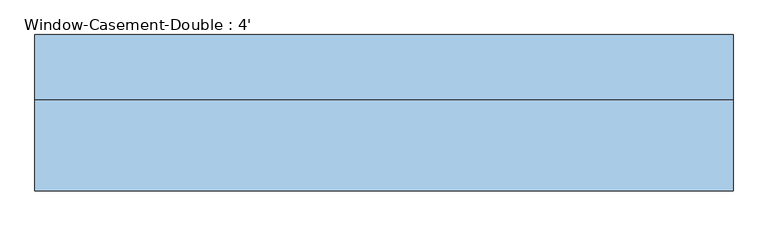
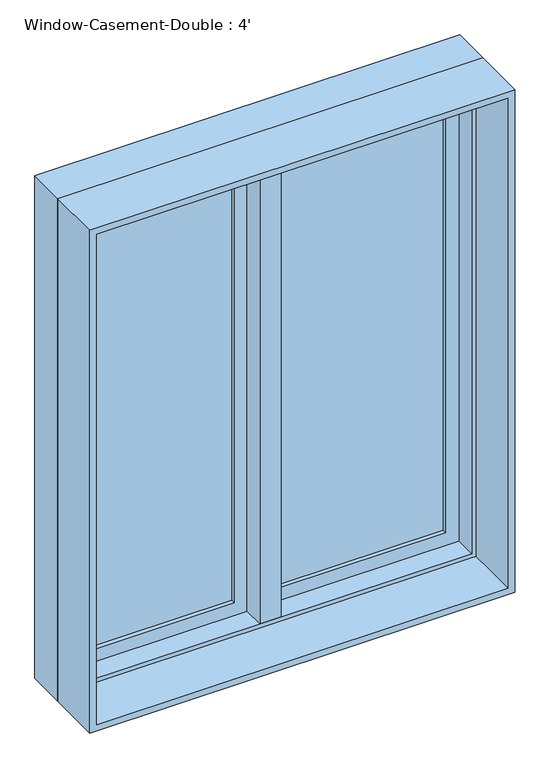
"""IFC4 building model written with IfcOpenShell, lengths in millimetres: window geometry, Window-Casement-Double : 4'."""

from ifc_helpers import new_model, si_unit, frame, origin, place, context, project, spatial, polyline, outline, extrude, faceted_brep, source, transform, mapped, element, save


def window_casement_double_4_a93ed6b4(model_context):
    return source(origin(), model_context, "Body", "SolidModel", [
        faceted_brep([(9.525, 146.05, 2425.7), (-9.525, 146.05, 2425.7), (-9.525, 95.25, 2425.7), (9.525, 95.25, 2425.7), (9.525, 146.05, 927.1), (9.525, 95.25, 927.1), (-9.525, 95.25, 927.1), (-9.525, 146.05, 927.1), (-9.525, 95.25, 946.15), (-9.525, 95.25, 2406.65), (-30.1625, 95.25, 946.15), (-30.1625, 95.25, 2406.65), (-30.1625, 31.75, 946.15), (-30.1625, 31.75, 2406.65), (30.1625, 31.75, 946.15), (30.1625, 31.75, 2406.65), (30.1625, 95.25, 946.15), (30.1625, 95.25, 2406.65), (9.525, 95.25, 946.15), (9.525, 95.25, 2406.65)], [[[0, 1, 2, 3]], [[4, 5, 6, 7]], [[1, 0, 4, 7]], [[2, 1, 7, 6, 8, 9]], [[9, 8, 10, 11]], [[11, 10, 12, 13]], [[13, 12, 14, 15]], [[15, 14, 16, 17]], [[17, 16, 18, 19]], [[0, 3, 19, 18, 5, 4]], [[18, 8, 6, 5]], [[9, 19, 3, 2]], [[8, 18, 16, 14, 12, 10]], [[19, 9, 11, 13, 15, 17]]]),
        extrude(outline(polyline([(-66.675, 127.0), (-66.675, 120.65), (-539.75, 120.65), (-539.75, 127.0), (-66.675, 127.0)])), frame((0.0, 0.0, 984.25), z_axis=(0.0, 0.0, 1.0), x_axis=(1.0, 0.0, 0.0)), (0.0, 0.0, 1.0), 1384.3),
        extrude(outline(polyline([(-539.75, 107.95), (-539.75, 114.3), (-66.675, 114.3), (-66.675, 107.95), (-539.75, 107.95)])), frame((0.0, 0.0, 984.25), z_axis=(0.0, 0.0, 1.0), x_axis=(1.0, 0.0, 0.0)), (0.0, 0.0, 1.0), 1384.3),
        extrude(outline(polyline([(539.75, 127.0), (539.75, 120.65), (66.675, 120.65), (66.675, 127.0), (539.75, 127.0)])), frame((0.0, 0.0, 984.25), z_axis=(0.0, 0.0, 1.0), x_axis=(1.0, 0.0, 0.0)), (0.0, 0.0, 1.0), 1384.3),
        extrude(outline(polyline([(66.675, 107.95), (66.675, 114.3), (539.75, 114.3), (539.75, 107.95), (66.675, 107.95)])), frame((0.0, 0.0, 984.25), z_axis=(0.0, 0.0, 1.0), x_axis=(1.0, 0.0, 0.0)), (0.0, 0.0, 1.0), 1384.3),
        extrude(outline(polyline([(2425.7, -596.9), (927.1, -596.9), (927.1, -9.525), (2425.7, -9.525), (2425.7, -596.9)]), holes=[polyline([(2368.55, -66.675), (984.25, -66.675), (984.25, -539.75), (2368.55, -539.75), (2368.55, -66.675)])]), frame((0.0, 95.25, 0.0), z_axis=(0.0, 1.0, 0.0), x_axis=(0.0, 0.0, 1.0)), (0.0, 0.0, 1.0), 44.45),
        extrude(outline(polyline([(927.1, 596.9), (2425.7, 596.9), (2425.7, 9.525), (927.1, 9.525), (927.1, 596.9)]), holes=[polyline([(984.25, 66.675), (2368.55, 66.675), (2368.55, 539.75), (984.25, 539.75), (984.25, 66.675)])]), frame((0.0, 95.25, 0.0), z_axis=(0.0, 1.0, 0.0), x_axis=(0.0, 0.0, 1.0)), (0.0, 0.0, 1.0), 44.45),
        extrude(outline(polyline([(2438.4, -609.6), (914.4, -609.6), (914.4, 609.6), (2438.4, 609.6), (2438.4, -609.6)]), holes=[polyline([(2419.35, 590.55), (933.45, 590.55), (933.45, -590.55), (2419.35, -590.55), (2419.35, 590.55)])]), frame((0.0, -127.0, 0.0), z_axis=(0.0, 1.0, 0.0), x_axis=(0.0, 0.0, 1.0)), (0.0, 0.0, 1.0), 158.75),
        faceted_brep([(577.85, 95.25, 2406.65), (577.85, 31.75, 2406.65), (-577.85, 31.75, 2406.65), (-577.85, 95.25, 2406.65), (596.9, 146.05, 2425.7), (596.9, 95.25, 2425.7), (-596.9, 95.25, 2425.7), (-596.9, 146.05, 2425.7), (609.6, 31.75, 2438.4), (609.6, 146.05, 2438.4), (-609.6, 146.05, 2438.4), (-609.6, 31.75, 2438.4), (-577.85, 31.75, 946.15), (-577.85, 95.25, 946.15), (-596.9, 95.25, 927.1), (-596.9, 146.05, 927.1), (-609.6, 146.05, 914.4), (-609.6, 31.75, 914.4), (577.85, 31.75, 946.15), (577.85, 95.25, 946.15), (596.9, 95.25, 927.1), (596.9, 146.05, 927.1), (609.6, 146.05, 914.4), (609.6, 31.75, 914.4)], [[[0, 1, 2, 3]], [[4, 5, 6, 7]], [[8, 9, 10, 11]], [[3, 2, 12, 13]], [[7, 6, 14, 15]], [[11, 10, 16, 17]], [[13, 12, 18, 19]], [[15, 14, 20, 21]], [[17, 16, 22, 23]], [[11, 17, 23, 8], [1, 18, 12, 2]], [[19, 18, 1, 0]], [[5, 20, 14, 6], [3, 13, 19, 0]], [[21, 20, 5, 4]], [[23, 22, 9, 8]], [[9, 22, 16, 10], [7, 15, 21, 4]]]),
    ])


if __name__ == "__main__":
    model = new_model("IFC4")
    model_context = context("Model", 3, world=origin())
    ifc_project = project(units=[si_unit("LENGTHUNIT", "METRE", prefix="MILLI")], contexts=[model_context])
    site = spatial("IfcSite", under=ifc_project)
    building = spatial("IfcBuilding", under=site)
    placement = place(None, origin())
    window_casement_double_4_shape = window_casement_double_4_a93ed6b4(model_context)
    element("IfcWindow", 1, ObjectType="Window-Casement-Double : 4'", at=placement, inside=building, context=model_context, shape_type="MappedRepresentation", body=[
        mapped(window_casement_double_4_shape, transform((0.0, 0.0, 0.0), x_axis=(1.0, 0.0, 0.0), y_axis=(0.0, 1.0, 0.0), z_axis=(0.0, 0.0, 1.0))),
    ])
    save(model, "model.ifc")

# Revit data of these elements
# Type "Window-Casement-Double : 4'"
#   Type Mark = "19"
#   Fire Rating = "0.5h"
#   Assembly Code = "B2020100"
#   Analytic Construction = "Double glazing - domestic"
#   Frame Extension [instance default] = 0' - 0 1/4"
#   Window Inset [instance default] = 0' - 0"
#   Wall Thickness [instance default] = 0' - 6"
#   Interior Wall Closure [instance default] = 0' - 2 1/4"
#   Half Width = 2' - 0"
#   Visual Light Transmittance = 0.81
#   Thermal Resistance (R) = 1.8146 (h·ft²·°F)/BTU
#   Solar Heat Gain Coefficient = 0.76
#   Rough Width = 4' - 0 1/2"
#   Rough Height = 5' - 0 1/2"
#   Height = 5' - 0"
#   Heat Transfer Coefficient (U) = 0.5511 BTU/(h·ft²·°F)
#   Exterior Wall Closure [instance default] = 0' - 1 1/4"
#   Extension Jamb [instance default] = 0' - 2 1/4"
#   Default Sill Height = 3' - 0"
#   Width = 4' - 0"
#   Muntin Visibility = yes
#   Interior Trim Visibility [instance default] = yes
#   Exterior Trim Visibility [instance default] = yes
#   Extension Jamb Visibility [instance default] = yes
#   Interior Trim Material = Wood - Stained
#   Muntin Pattern = Muntin Pattern_2x2 : Muntin Pattern_2x2
#   Interior Trim = Trim-Window-Interior-Flat : Picture Frame
#   Interior Frame Material = Wood - Stained
#   Glass Panel Material = Glass
#   Exterior Trim Material = Clad - White
#   Exterior Trim = Trim-Window-Exterior-Flat : with Sill
#   Exterior Frame Material = Clad - White
#   Wall Closure = (empty or 0)
# Element 1 (IfcWindow, "Window-Casement-Double : 4'")
#   Wall Thickness = 0' - 10"
#   Extension Jamb = 0' - 6 1/4"
#   Materials on its faces: "Wood - Stained", "Glass", "Clad - White"
# Materials
#   "Wood - Stained": class "Wood", colour RGB 224 178 126, transparency 0, Cost = 0
#   "Glass": class "Glass", colour RGB 0 128 192, transparency 0.75, Description = "Soda Lime Glass", Cost = 0
#   "Clad - White": class "Wood", colour RGB 242 242 238, transparency 0, Cost = 0
